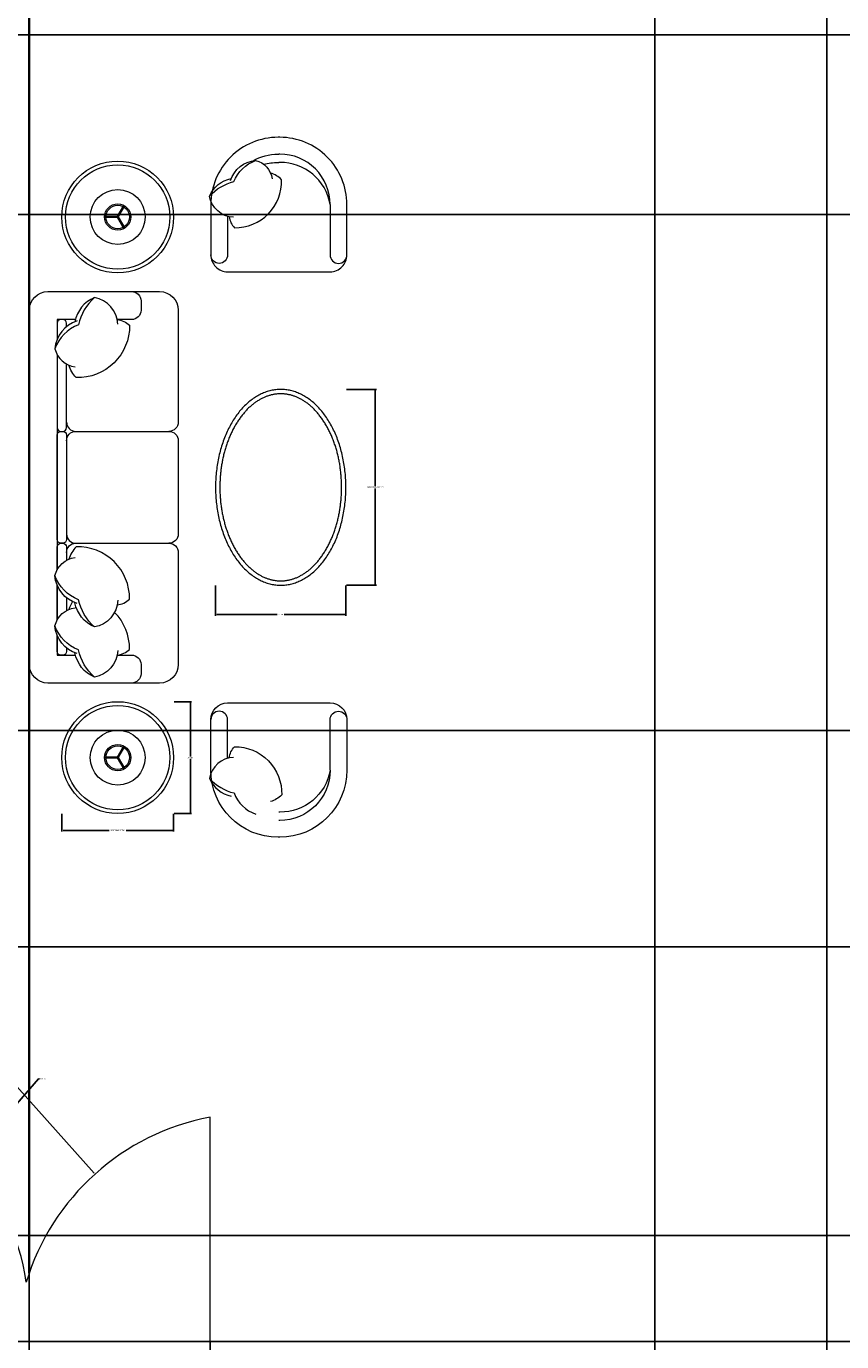
# Model space of a CAD drawing. Units: inches. Extents: x 1861 to 2564, y 1482 to 2317.
# Tile 8 of 11: x 2217 to 2339, y 1853 to 2051. Entities that reach past the tile are written whole.
import ezdxf

# ---------------------------------------------------------------- set-up
doc = ezdxf.new("R2010")
doc.units = ezdxf.units.IN
for name, color, linetype, lineweight in [('A-ANNO-DIMS', 2, 'Continuous', 18), ('A-DOOR', 3, 'Continuous', 18), ('A-FURN', 8, 'Continuous', 13), ('A-WALL', 7, 'Continuous', 35)]:
    doc.layers.add(name, color=color, linetype=linetype, lineweight=lineweight)
doc.styles.get("Standard").update_dxf_attribs({"font": 'arial.ttf'})
doc.dimstyles.get("Standard").update_dxf_attribs({"dimtxt": 0.18, "dimasz": 0.18, "dimexe": 0.18, "dimexo": 0.0625, "dimgap": 0.09, "dimtad": 0, "dimtih": 1, "dimtoh": 1, "dimdec": 4, "dimzin": 0, "dimdsep": 46, "dimtxsty": 'Standard', "dimcen": 0.09, "dimadec": 0, "dimazin": 0, "dimtfac": 1, "dimtdec": 4, "dimtofl": 0, "dimtmove": 0, "dimatfit": 3, "dimfxl": 1, "dimtolj": 1, "dimtzin": 0, "dimarcsym": 0})

# ---------------------------------------------------------------- blocks, each defined once
blk = doc.blocks.new('TABLE-SIDE-ROUND')
at = {"ltscale": 0.03}
for p, q in [((8.34, 8.45), (9.33, 10.16)), ((8.49, 8.36), (9.48, 10.08)), ((8.41, 8.5), (6.44, 8.5)), ((8.41, 8.32), (6.44, 8.32)), ((8.34, 8.36), (9.33, 6.65)), ((8.49, 8.45), (9.48, 6.74))]:
    blk.add_line(p, q, dxfattribs=at)
for radius in [8.41, 4.13, 1.98, 1.77]:
    blk.add_circle((8.41, 8.41), radius, dxfattribs=at)
blk.add_circle((8.41, 8.41), 7.85)
blk = doc.blocks.new('CHAIR-LOUNGE')
at = {"ltscale": 0.03}
blk.add_lwpolyline([(10.44, 0), (18.15, 0, 0.414214), (20.68, 2.53), (20.68, 10.11, 0.414214), (10.57, 20.22), (10.44, 20.22), (10.32, 20.22, 0.414214), (0.21, 10.11), (0.21, 2.53, 0.414214), (2.73, 0), (10.44, 0)], format="xyb", dxfattribs=at)
for points in [[(0, 11.38, -0.14773), (3.69, 13.56, -0.213343), (6.95, 16.74, -0.178662)], [(3.18, 13.73, -0.306663), (6.95, 16.74, -0.30633), (9.42, 13.99, 0.872847)], [(6.55, 16.69, -0.130591), (10.32, 17.69), (10.44, 17.69)], [(8.16, 16.16, -0.072384), (10.32, 16.43), (10.44, 16.43)], [(18.15, 10.11, 0.414214), (10.57, 17.69), (10.44, 17.69)], [(18.15, 10.11, 0.372719), (10.57, 16.43), (10.44, 16.43)], [(3.62, 8.2, -0.356772), (0, 11.38, -0.249542), (3.28, 14.01, 9.61688)], [(2.98, 8.28, 0.165541), (3.77, 6.61, 0.425989), (10.86, 13.85, 0.121523), (9.18, 14.84, -7.115464)], [(18.15, 10.11), (18.15, 2.53, 0.414214), (19.42, 1.26), (19.42, 1.26, 0.414214), (20.68, 2.53)], [(2.73, 8.34), (2.73, 2.53, -0.414214), (1.47, 1.26), (1.47, 1.26, -0.414214), (0.21, 2.53)]]:
    blk.add_lwpolyline(points, format="xyb")
blk = doc.blocks.new('TABLE-COFFEE-OVAL')
at = {"ltscale": 0.03}
blk.add_polyline3d([(9.81, 29.44, 0), (9.63, 29.44, 0), (9.44, 29.43, 0), (9.26, 29.41, 0), (9.07, 29.4, 0), (8.89, 29.37, 0), (8.7, 29.34, 0), (8.52, 29.31, 0), (8.33, 29.27, 0), (8.15, 29.23, 0), (7.97, 29.18, 0), (7.79, 29.12, 0), (7.6, 29.06, 0), (7.42, 28.99, 0), (7.24, 28.92, 0), (7.07, 28.85, 0), (6.89, 28.77, 0), (6.71, 28.68, 0), (6.54, 28.59, 0), (6.36, 28.5, 0), (6.19, 28.4, 0), (6.02, 28.29, 0), (5.85, 28.18, 0), (5.68, 28.07, 0), (5.51, 27.95, 0), (5.34, 27.82, 0), (5.18, 27.69, 0), (5.02, 27.56, 0), (4.85, 27.42, 0), (4.69, 27.28, 0), (4.54, 27.13, 0), (4.38, 26.98, 0), (4.23, 26.82, 0), (4.08, 26.66, 0), (3.93, 26.49, 0), (3.78, 26.33, 0), (3.63, 26.15, 0), (3.49, 25.97, 0), (3.35, 25.79, 0), (3.21, 25.61, 0), (3.08, 25.42, 0), (2.94, 25.23, 0), (2.81, 25.03, 0), (2.68, 24.83, 0), (2.56, 24.62, 0), (2.43, 24.42, 0), (2.31, 24.2, 0), (2.19, 23.99, 0), (2.08, 23.77, 0), (1.96, 23.55, 0), (1.85, 23.33, 0), (1.75, 23.1, 0), (1.64, 22.87, 0), (1.54, 22.63, 0), (1.44, 22.4, 0), (1.35, 22.16, 0), (1.26, 21.92, 0), (1.17, 21.67, 0), (1.08, 21.43, 0), (1, 21.18, 0), (0.92, 20.93, 0), (0.84, 20.67, 0), (0.77, 20.42, 0), (0.7, 20.16, 0), (0.63, 19.9, 0), (0.57, 19.64, 0), (0.51, 19.37, 0), (0.45, 19.11, 0), (0.39, 18.84, 0), (0.34, 18.57, 0), (0.3, 18.31, 0), (0.25, 18.03, 0), (0.21, 17.76, 0), (0.18, 17.49, 0), (0.14, 17.22, 0), (0.11, 16.94, 0), (0.09, 16.66, 0), (0.07, 16.39, 0), (0.05, 16.11, 0), (0.03, 15.83, 0), (0.02, 15.56, 0), (0.01, 15.28, 0), (0, 15, 0), (0, 14.72, 0), (0, 14.44, 0), (0.01, 14.16, 0), (0.02, 13.89, 0), (0.03, 13.61, 0), (0.05, 13.33, 0), (0.07, 13.05, 0), (0.09, 12.78, 0), (0.11, 12.5, 0), (0.14, 12.23, 0), (0.18, 11.95, 0), (0.21, 11.68, 0), (0.25, 11.41, 0), (0.3, 11.14, 0), (0.34, 10.87, 0), (0.39, 10.6, 0), (0.45, 10.33, 0), (0.51, 10.07, 0), (0.57, 9.8, 0), (0.63, 9.54, 0), (0.7, 9.28, 0), (0.77, 9.02, 0), (0.84, 8.77, 0), (0.92, 8.52, 0), (1, 8.26, 0), (1.08, 8.01, 0), (1.17, 7.77, 0), (1.26, 7.52, 0), (1.35, 7.28, 0), (1.44, 7.04, 0), (1.54, 6.81, 0), (1.64, 6.57, 0), (1.75, 6.34, 0), (1.85, 6.12, 0), (1.96, 5.89, 0), (2.08, 5.67, 0), (2.19, 5.45, 0), (2.31, 5.24, 0), (2.43, 5.03, 0), (2.56, 4.82, 0), (2.68, 4.61, 0), (2.81, 4.41, 0), (2.94, 4.22, 0), (3.08, 4.02, 0), (3.21, 3.83, 0), (3.35, 3.65, 0), (3.49, 3.47, 0), (3.63, 3.29, 0), (3.78, 3.12, 0), (3.93, 2.95, 0), (4.08, 2.78, 0), (4.23, 2.62, 0), (4.38, 2.46, 0), (4.54, 2.31, 0), (4.69, 2.17, 0), (4.85, 2.02, 0), (5.02, 1.88, 0), (5.18, 1.75, 0), (5.34, 1.62, 0), (5.51, 1.5, 0), (5.68, 1.38, 0), (5.85, 1.26, 0), (6.02, 1.15, 0), (6.19, 1.05, 0), (6.36, 0.94, 0), (6.54, 0.85, 0), (6.71, 0.76, 0), (6.89, 0.67, 0), (7.07, 0.59, 0), (7.24, 0.52, 0), (7.42, 0.45, 0), (7.6, 0.38, 0), (7.79, 0.32, 0), (7.97, 0.27, 0), (8.15, 0.22, 0), (8.33, 0.17, 0), (8.52, 0.13, 0), (8.7, 0.1, 0), (8.89, 0.07, 0), (9.07, 0.05, 0), (9.26, 0.03, 0), (9.44, 0.01, 0), (9.63, 0.01, 0), (9.81, 0, 0), (10, 0.01, 0), (10.18, 0.01, 0), (10.37, 0.03, 0), (10.56, 0.05, 0), (10.74, 0.07, 0), (10.93, 0.1, 0), (11.11, 0.13, 0), (11.29, 0.17, 0), (11.48, 0.22, 0), (11.66, 0.27, 0), (11.84, 0.32, 0), (12.02, 0.38, 0), (12.2, 0.45, 0), (12.38, 0.52, 0), (12.56, 0.59, 0), (12.74, 0.67, 0), (12.92, 0.76, 0), (13.09, 0.85, 0), (13.27, 0.94, 0), (13.44, 1.05, 0), (13.61, 1.15, 0), (13.78, 1.26, 0), (13.95, 1.38, 0), (14.12, 1.5, 0), (14.28, 1.62, 0), (14.45, 1.75, 0), (14.61, 1.88, 0), (14.77, 2.02, 0), (14.93, 2.17, 0), (15.09, 2.31, 0), (15.25, 2.46, 0), (15.4, 2.62, 0), (15.55, 2.78, 0), (15.7, 2.95, 0), (15.85, 3.12, 0), (15.99, 3.29, 0), (16.14, 3.47, 0), (16.28, 3.65, 0), (16.42, 3.83, 0), (16.55, 4.02, 0), (16.69, 4.22, 0), (16.82, 4.41, 0), (16.95, 4.61, 0), (17.07, 4.82, 0), (17.2, 5.03, 0), (17.32, 5.24, 0), (17.43, 5.45, 0), (17.55, 5.67, 0), (17.66, 5.89, 0), (17.77, 6.12, 0), (17.88, 6.34, 0), (17.98, 6.57, 0), (18.09, 6.81, 0), (18.18, 7.04, 0), (18.28, 7.28, 0), (18.37, 7.52, 0), (18.46, 7.77, 0), (18.55, 8.01, 0), (18.63, 8.26, 0), (18.71, 8.52, 0), (18.79, 8.77, 0), (18.86, 9.02, 0), (18.93, 9.28, 0), (19, 9.54, 0), (19.06, 9.8, 0), (19.12, 10.07, 0), (19.18, 10.33, 0), (19.23, 10.6, 0), (19.28, 10.87, 0), (19.33, 11.14, 0), (19.37, 11.41, 0), (19.41, 11.68, 0), (19.45, 11.95, 0), (19.48, 12.23, 0), (19.51, 12.5, 0), (19.54, 12.78, 0), (19.56, 13.05, 0), (19.58, 13.33, 0), (19.6, 13.61, 0), (19.61, 13.89, 0), (19.62, 14.16, 0), (19.62, 14.44, 0), (19.63, 14.72, 0), (19.62, 15, 0), (19.62, 15.28, 0), (19.61, 15.56, 0), (19.6, 15.83, 0), (19.58, 16.11, 0), (19.56, 16.39, 0), (19.54, 16.66, 0), (19.51, 16.94, 0), (19.48, 17.22, 0), (19.45, 17.49, 0), (19.41, 17.76, 0), (19.37, 18.03, 0), (19.33, 18.31, 0), (19.28, 18.57, 0), (19.23, 18.84, 0), (19.18, 19.11, 0), (19.12, 19.37, 0), (19.06, 19.64, 0), (19, 19.9, 0), (18.93, 20.16, 0), (18.86, 20.42, 0), (18.79, 20.67, 0), (18.71, 20.93, 0), (18.63, 21.18, 0), (18.55, 21.43, 0), (18.46, 21.67, 0), (18.37, 21.92, 0), (18.28, 22.16, 0), (18.18, 22.4, 0), (18.09, 22.63, 0), (17.98, 22.87, 0), (17.88, 23.1, 0), (17.77, 23.33, 0), (17.66, 23.55, 0), (17.55, 23.77, 0), (17.43, 23.99, 0), (17.32, 24.2, 0), (17.2, 24.42, 0), (17.07, 24.62, 0), (16.95, 24.83, 0), (16.82, 25.03, 0), (16.69, 25.23, 0), (16.55, 25.42, 0), (16.42, 25.61, 0), (16.28, 25.79, 0), (16.14, 25.97, 0), (15.99, 26.15, 0), (15.85, 26.33, 0), (15.7, 26.49, 0), (15.55, 26.66, 0), (15.4, 26.82, 0), (15.25, 26.98, 0), (15.09, 27.13, 0), (14.93, 27.28, 0), (14.77, 27.42, 0), (14.61, 27.56, 0), (14.45, 27.69, 0), (14.28, 27.82, 0), (14.12, 27.95, 0), (13.95, 28.07, 0), (13.78, 28.18, 0), (13.61, 28.29, 0), (13.44, 28.4, 0), (13.27, 28.5, 0), (13.09, 28.59, 0), (12.92, 28.68, 0), (12.74, 28.77, 0), (12.56, 28.85, 0), (12.38, 28.92, 0), (12.2, 28.99, 0), (12.02, 29.06, 0), (11.84, 29.12, 0), (11.66, 29.18, 0), (11.48, 29.23, 0), (11.29, 29.27, 0), (11.11, 29.31, 0), (10.93, 29.34, 0), (10.74, 29.37, 0), (10.56, 29.4, 0), (10.37, 29.41, 0), (10.18, 29.43, 0), (10, 29.44, 0), (9.81, 29.44, 0)], dxfattribs=at)
blk.add_polyline3d([(9.81, 28.78, 0), (9.71, 28.78, 0), (9.61, 28.78, 0), (9.51, 28.78, 0), (9.41, 28.77, 0), (9.31, 28.76, 0), (9.2, 28.75, 0), (9.1, 28.74, 0), (9, 28.73, 0), (8.89, 28.71, 0), (8.79, 28.69, 0), (8.69, 28.68, 0), (8.58, 28.65, 0), (8.48, 28.63, 0), (8.37, 28.61, 0), (8.27, 28.58, 0), (8.16, 28.55, 0), (8.05, 28.52, 0), (7.95, 28.49, 0), (7.84, 28.45, 0), (7.73, 28.41, 0), (7.63, 28.37, 0), (7.52, 28.33, 0), (7.41, 28.29, 0), (7.31, 28.24, 0), (7.2, 28.19, 0), (7.09, 28.14, 0), (6.98, 28.09, 0), (6.88, 28.03, 0), (6.77, 27.97, 0), (6.66, 27.91, 0), (6.55, 27.85, 0), (6.45, 27.79, 0), (6.34, 27.72, 0), (6.23, 27.65, 0), (6.13, 27.58, 0), (6.02, 27.51, 0), (5.92, 27.43, 0), (5.81, 27.36, 0), (5.71, 27.28, 0), (5.6, 27.19, 0), (5.5, 27.11, 0), (5.39, 27.02, 0), (5.29, 26.93, 0), (5.19, 26.84, 0), (5.09, 26.75, 0), (4.98, 26.65, 0), (4.88, 26.55, 0), (4.78, 26.45, 0), (4.68, 26.34, 0), (4.58, 26.24, 0), (4.49, 26.13, 0), (4.39, 26.02, 0), (4.29, 25.91, 0), (4.2, 25.79, 0), (4.1, 25.68, 0), (4.01, 25.56, 0), (3.91, 25.44, 0), (3.82, 25.32, 0), (3.73, 25.19, 0), (3.64, 25.07, 0), (3.55, 24.94, 0), (3.46, 24.81, 0), (3.37, 24.68, 0), (3.29, 24.54, 0), (3.2, 24.41, 0), (3.12, 24.27, 0), (3.03, 24.13, 0), (2.95, 23.99, 0), (2.87, 23.85, 0), (2.79, 23.71, 0), (2.71, 23.56, 0), (2.63, 23.41, 0), (2.56, 23.27, 0), (2.48, 23.12, 0), (2.41, 22.97, 0), (2.34, 22.81, 0), (2.27, 22.66, 0), (2.2, 22.51, 0), (2.13, 22.35, 0), (2.07, 22.19, 0), (2, 22.04, 0), (1.94, 21.88, 0), (1.88, 21.72, 0), (1.82, 21.55, 0), (1.76, 21.39, 0), (1.7, 21.23, 0), (1.65, 21.07, 0), (1.6, 20.9, 0), (1.54, 20.74, 0), (1.49, 20.58, 0), (1.44, 20.41, 0), (1.4, 20.25, 0), (1.35, 20.08, 0), (1.31, 19.92, 0), (1.26, 19.75, 0), (1.22, 19.59, 0), (1.18, 19.42, 0), (1.15, 19.25, 0), (1.11, 19.09, 0), (1.07, 18.92, 0), (1.04, 18.75, 0), (1.01, 18.58, 0), (0.98, 18.42, 0), (0.95, 18.25, 0), (0.92, 18.08, 0), (0.89, 17.91, 0), (0.87, 17.74, 0), (0.84, 17.57, 0), (0.82, 17.4, 0), (0.8, 17.23, 0), (0.78, 17.06, 0), (0.76, 16.89, 0), (0.75, 16.72, 0), (0.73, 16.55, 0), (0.72, 16.38, 0), (0.71, 16.21, 0), (0.7, 16.04, 0), (0.69, 15.87, 0), (0.68, 15.7, 0), (0.67, 15.53, 0), (0.67, 15.36, 0), (0.66, 15.19, 0), (0.66, 15.02, 0), (0.66, 14.85, 0), (0.66, 14.68, 0), (0.66, 14.51, 0), (0.66, 14.34, 0), (0.66, 14.17, 0), (0.67, 14, 0), (0.67, 13.82, 0), (0.68, 13.65, 0), (0.69, 13.48, 0), (0.7, 13.31, 0), (0.71, 13.14, 0), (0.73, 12.97, 0), (0.74, 12.8, 0), (0.76, 12.63, 0), (0.77, 12.46, 0), (0.79, 12.29, 0), (0.81, 12.12, 0), (0.83, 11.95, 0), (0.86, 11.78, 0), (0.88, 11.62, 0), (0.91, 11.45, 0), (0.93, 11.28, 0), (0.96, 11.11, 0), (0.99, 10.94, 0), (1.02, 10.77, 0), (1.06, 10.61, 0), (1.09, 10.44, 0), (1.13, 10.27, 0), (1.16, 10.1, 0), (1.2, 9.94, 0), (1.24, 9.77, 0), (1.29, 9.61, 0), (1.33, 9.44, 0), (1.37, 9.28, 0), (1.42, 9.11, 0), (1.47, 8.95, 0), (1.52, 8.78, 0), (1.57, 8.62, 0), (1.62, 8.46, 0), (1.68, 8.29, 0), (1.73, 8.13, 0), (1.79, 7.97, 0), (1.85, 7.81, 0), (1.91, 7.65, 0), (1.97, 7.49, 0), (2.03, 7.33, 0), (2.1, 7.17, 0), (2.17, 7.01, 0), (2.23, 6.86, 0), (2.3, 6.7, 0), (2.37, 6.55, 0), (2.45, 6.4, 0), (2.52, 6.25, 0), (2.6, 6.1, 0), (2.67, 5.95, 0), (2.75, 5.81, 0), (2.83, 5.66, 0), (2.91, 5.52, 0), (2.99, 5.38, 0), (3.07, 5.24, 0), (3.16, 5.1, 0), (3.24, 4.97, 0), (3.33, 4.83, 0), (3.42, 4.7, 0), (3.5, 4.57, 0), (3.59, 4.44, 0), (3.68, 4.31, 0), (3.77, 4.19, 0), (3.87, 4.06, 0), (3.96, 3.94, 0), (4.05, 3.82, 0), (4.15, 3.71, 0), (4.24, 3.59, 0), (4.34, 3.48, 0), (4.44, 3.37, 0), (4.53, 3.26, 0), (4.63, 3.15, 0), (4.73, 3.04, 0), (4.83, 2.94, 0), (4.93, 2.84, 0), (5.03, 2.74, 0), (5.14, 2.65, 0), (5.24, 2.56, 0), (5.34, 2.47, 0), (5.44, 2.38, 0), (5.55, 2.29, 0), (5.65, 2.21, 0), (5.76, 2.13, 0), (5.86, 2.05, 0), (5.97, 1.97, 0), (6.07, 1.9, 0), (6.18, 1.82, 0), (6.29, 1.75, 0), (6.39, 1.69, 0), (6.5, 1.62, 0), (6.61, 1.56, 0), (6.72, 1.5, 0), (6.82, 1.44, 0), (6.93, 1.38, 0), (7.04, 1.33, 0), (7.14, 1.28, 0), (7.25, 1.23, 0), (7.36, 1.18, 0), (7.47, 1.13, 0), (7.57, 1.09, 0), (7.68, 1.05, 0), (7.79, 1.01, 0), (7.89, 0.97, 0), (8, 0.94, 0), (8.11, 0.91, 0), (8.21, 0.88, 0), (8.32, 0.85, 0), (8.42, 0.82, 0), (8.53, 0.8, 0), (8.63, 0.78, 0), (8.74, 0.76, 0), (8.84, 0.74, 0), (8.95, 0.72, 0), (9.05, 0.71, 0), (9.15, 0.69, 0), (9.26, 0.68, 0), (9.36, 0.68, 0), (9.46, 0.67, 0), (9.56, 0.66, 0), (9.66, 0.66, 0), (9.76, 0.66, 0), (9.86, 0.66, 0), (9.96, 0.66, 0), (10.07, 0.66, 0), (10.17, 0.67, 0), (10.27, 0.68, 0), (10.37, 0.68, 0), (10.47, 0.69, 0), (10.58, 0.71, 0), (10.68, 0.72, 0), (10.78, 0.74, 0), (10.89, 0.76, 0), (10.99, 0.78, 0), (11.1, 0.8, 0), (11.2, 0.82, 0), (11.31, 0.85, 0), (11.41, 0.88, 0), (11.52, 0.91, 0), (11.63, 0.94, 0), (11.73, 0.97, 0), (11.84, 1.01, 0), (11.95, 1.05, 0), (12.05, 1.09, 0), (12.16, 1.13, 0), (12.27, 1.18, 0), (12.37, 1.23, 0), (12.48, 1.28, 0), (12.59, 1.33, 0), (12.7, 1.38, 0), (12.8, 1.44, 0), (12.91, 1.5, 0), (13.02, 1.56, 0), (13.13, 1.62, 0), (13.23, 1.69, 0), (13.34, 1.75, 0), (13.45, 1.82, 0), (13.55, 1.9, 0), (13.66, 1.97, 0), (13.76, 2.05, 0), (13.87, 2.13, 0), (13.97, 2.21, 0), (14.08, 2.29, 0), (14.18, 2.38, 0), (14.29, 2.47, 0), (14.39, 2.56, 0), (14.49, 2.65, 0), (14.59, 2.74, 0), (14.69, 2.84, 0), (14.79, 2.94, 0), (14.89, 3.04, 0), (14.99, 3.15, 0), (15.09, 3.26, 0), (15.19, 3.37, 0), (15.29, 3.48, 0), (15.38, 3.59, 0), (15.48, 3.71, 0), (15.57, 3.82, 0), (15.67, 3.94, 0), (15.76, 4.06, 0), (15.85, 4.19, 0), (15.94, 4.31, 0), (16.03, 4.44, 0), (16.12, 4.57, 0), (16.21, 4.7, 0), (16.3, 4.83, 0), (16.38, 4.97, 0), (16.47, 5.1, 0), (16.55, 5.24, 0), (16.64, 5.38, 0), (16.72, 5.52, 0), (16.8, 5.66, 0), (16.88, 5.81, 0), (16.95, 5.95, 0), (17.03, 6.1, 0), (17.11, 6.25, 0), (17.18, 6.4, 0), (17.25, 6.55, 0), (17.32, 6.7, 0), (17.39, 6.86, 0), (17.46, 7.01, 0), (17.53, 7.17, 0), (17.59, 7.33, 0), (17.66, 7.49, 0), (17.72, 7.65, 0), (17.78, 7.81, 0), (17.84, 7.97, 0), (17.9, 8.13, 0), (17.95, 8.29, 0), (18.01, 8.46, 0), (18.06, 8.62, 0), (18.11, 8.78, 0), (18.16, 8.95, 0), (18.21, 9.11, 0), (18.25, 9.28, 0), (18.3, 9.44, 0), (18.34, 9.61, 0), (18.38, 9.77, 0), (18.42, 9.94, 0), (18.46, 10.1, 0), (18.5, 10.27, 0), (18.54, 10.44, 0), (18.57, 10.61, 0), (18.6, 10.77, 0), (18.63, 10.94, 0), (18.66, 11.11, 0), (18.69, 11.28, 0), (18.72, 11.45, 0), (18.75, 11.62, 0), (18.77, 11.78, 0), (18.79, 11.95, 0), (18.81, 12.12, 0), (18.83, 12.29, 0), (18.85, 12.46, 0), (18.87, 12.63, 0), (18.89, 12.8, 0), (18.9, 12.97, 0), (18.91, 13.14, 0), (18.93, 13.31, 0), (18.94, 13.48, 0), (18.95, 13.65, 0), (18.95, 13.82, 0), (18.96, 14, 0), (18.96, 14.17, 0), (18.97, 14.34, 0), (18.97, 14.51, 0), (18.97, 14.68, 0), (18.97, 14.85, 0), (18.97, 15.02, 0), (18.97, 15.19, 0), (18.96, 15.36, 0), (18.96, 15.53, 0), (18.95, 15.7, 0), (18.94, 15.87, 0), (18.93, 16.04, 0), (18.92, 16.21, 0), (18.91, 16.38, 0), (18.89, 16.55, 0), (18.88, 16.72, 0), (18.86, 16.89, 0), (18.84, 17.06, 0), (18.83, 17.23, 0), (18.8, 17.4, 0), (18.78, 17.57, 0), (18.76, 17.74, 0), (18.73, 17.91, 0), (18.71, 18.08, 0), (18.68, 18.25, 0), (18.65, 18.42, 0), (18.62, 18.58, 0), (18.59, 18.75, 0), (18.55, 18.92, 0), (18.52, 19.09, 0), (18.48, 19.25, 0), (18.44, 19.42, 0), (18.4, 19.59, 0), (18.36, 19.75, 0), (18.32, 19.92, 0), (18.28, 20.08, 0), (18.23, 20.25, 0), (18.18, 20.41, 0), (18.13, 20.58, 0), (18.08, 20.74, 0), (18.03, 20.9, 0), (17.98, 21.07, 0), (17.92, 21.23, 0), (17.87, 21.39, 0), (17.81, 21.55, 0), (17.75, 21.72, 0), (17.69, 21.88, 0), (17.62, 22.04, 0), (17.56, 22.19, 0), (17.49, 22.35, 0), (17.43, 22.51, 0), (17.36, 22.66, 0), (17.29, 22.81, 0), (17.22, 22.97, 0), (17.14, 23.12, 0), (17.07, 23.27, 0), (16.99, 23.41, 0), (16.92, 23.56, 0), (16.84, 23.71, 0), (16.76, 23.85, 0), (16.68, 23.99, 0), (16.59, 24.13, 0), (16.51, 24.27, 0), (16.43, 24.41, 0), (16.34, 24.54, 0), (16.26, 24.68, 0), (16.17, 24.81, 0), (16.08, 24.94, 0), (15.99, 25.07, 0), (15.9, 25.19, 0), (15.81, 25.32, 0), (15.71, 25.44, 0), (15.62, 25.56, 0), (15.53, 25.68, 0), (15.43, 25.79, 0), (15.34, 25.91, 0), (15.24, 26.02, 0), (15.14, 26.13, 0), (15.04, 26.24, 0), (14.94, 26.34, 0), (14.84, 26.45, 0), (14.74, 26.55, 0), (14.64, 26.65, 0), (14.54, 26.75, 0), (14.44, 26.84, 0), (14.34, 26.93, 0), (14.23, 27.02, 0), (14.13, 27.11, 0), (14.03, 27.19, 0), (13.92, 27.28, 0), (13.82, 27.36, 0), (13.71, 27.43, 0), (13.61, 27.51, 0), (13.5, 27.58, 0), (13.39, 27.65, 0), (13.29, 27.72, 0), (13.18, 27.79, 0), (13.07, 27.85, 0), (12.97, 27.91, 0), (12.86, 27.97, 0), (12.75, 28.03, 0), (12.64, 28.09, 0), (12.54, 28.14, 0), (12.43, 28.19, 0), (12.32, 28.24, 0), (12.21, 28.29, 0), (12.11, 28.33, 0), (12, 28.37, 0), (11.89, 28.41, 0), (11.79, 28.45, 0), (11.68, 28.49, 0), (11.57, 28.52, 0), (11.47, 28.55, 0), (11.36, 28.58, 0), (11.26, 28.61, 0), (11.15, 28.63, 0), (11.05, 28.65, 0), (10.94, 28.68, 0), (10.84, 28.69, 0), (10.73, 28.71, 0), (10.63, 28.73, 0), (10.53, 28.74, 0), (10.42, 28.75, 0), (10.32, 28.76, 0), (10.22, 28.77, 0), (10.12, 28.78, 0), (10.01, 28.78, 0), (9.91, 28.78, 0), (9.81, 28.78, 0)])
blk = doc.blocks.new('*D28')
at = {"layer": 'A-ANNO-DIMS', "color": 0, "lineweight": -2, "transparency": 16777216}
for p, q in [((2222.15, 1932.74), (2222.15, 1930.1)), ((2238.96, 1932.74), (2238.96, 1930.1)), ((2222.33, 1930.28), (2229.27, 1930.28)), ((2238.78, 1930.28), (2231.84, 1930.28))]:
    blk.add_line(p, q, dxfattribs=at)
at = {"layer": 'A-ANNO-DIMS', "color": 0, "transparency": 16777216}
for points in [[(2222.33, 1930.31), (2222.33, 1930.25), (2222.15, 1930.28)], [(2238.78, 1930.31), (2238.78, 1930.25), (2238.96, 1930.28)]]:
    blk.add_solid(points, dxfattribs=at)
at = {"layer": 'Defpoints', "color": 0, "transparency": 16777216}
for p in [(2222.15, 1932.8), (2238.96, 1932.8), (2238.96, 1930.28)]:
    blk.add_point(p, dxfattribs=at)
at = {"layer": 'A-ANNO-DIMS', "color": 0, "transparency": 16777216, "insert": (2230.55, 1930.28), "char_height": 0.18, "attachment_point": 5}
blk.add_mtext('\\A1;SIDE TABLE 17 TYP.', dxfattribs=at)
blk = doc.blocks.new('*D29')
at = {"layer": 'A-ANNO-DIMS', "color": 0, "lineweight": -2, "transparency": 16777216}
for p, q in [((2239.03, 1949.62), (2241.67, 1949.62)), ((2241.49, 1949.44), (2241.49, 1941.39)), ((2241.49, 1932.98), (2241.49, 1941.03)), ((2239.03, 1932.8), (2241.67, 1932.8))]:
    blk.add_line(p, q, dxfattribs=at)
at = {"layer": 'A-ANNO-DIMS', "color": 0, "transparency": 16777216}
for points in [[(2241.46, 1949.44), (2241.52, 1949.44), (2241.49, 1949.62)], [(2241.46, 1932.98), (2241.52, 1932.98), (2241.49, 1932.8)]]:
    blk.add_solid(points, dxfattribs=at)
at = {"layer": 'Defpoints', "color": 0, "transparency": 16777216}
for p in [(2238.96, 1949.62), (2241.49, 1949.62), (2238.96, 1932.8)]:
    blk.add_point(p, dxfattribs=at)
at = {"layer": 'A-ANNO-DIMS', "color": 0, "transparency": 16777216, "insert": (2241.49, 1941.21), "char_height": 0.18, "attachment_point": 5}
blk.add_mtext('\\A1;17 TYP.', dxfattribs=at)
blk = doc.blocks.new('*D30')
at = {"layer": 'A-ANNO-DIMS', "color": 0, "lineweight": -2, "transparency": 16777216}
for p, q in [((2264.96, 1996.58), (2269.49, 1996.58)), ((2269.31, 1996.4), (2269.31, 1982.04)), ((2269.31, 1967.32), (2269.31, 1981.68)), ((2264.96, 1967.14), (2269.49, 1967.14))]:
    blk.add_line(p, q, dxfattribs=at)
at = {"layer": 'A-ANNO-DIMS', "color": 0, "transparency": 16777216}
for points in [[(2269.28, 1996.4), (2269.34, 1996.4), (2269.31, 1996.58)], [(2269.28, 1967.32), (2269.34, 1967.32), (2269.31, 1967.14)]]:
    blk.add_solid(points, dxfattribs=at)
at = {"layer": 'Defpoints', "color": 0, "transparency": 16777216}
for p in [(2264.9, 1996.58), (2269.31, 1996.58), (2264.9, 1967.14)]:
    blk.add_point(p, dxfattribs=at)
at = {"layer": 'A-ANNO-DIMS', "color": 0, "transparency": 16777216, "insert": (2269.31, 1981.86), "char_height": 0.18, "attachment_point": 5}
blk.add_mtext('\\A1;COFFEE TABLE 29 TYP.', dxfattribs=at)
blk = doc.blocks.new('*D31')
at = {"layer": 'A-ANNO-DIMS', "color": 0, "lineweight": -2, "transparency": 16777216}
for p, q in [((2245.27, 1967.08), (2245.27, 1962.55)), ((2264.9, 1967.08), (2264.9, 1962.55)), ((2245.45, 1962.73), (2254.55, 1962.73)), ((2264.72, 1962.73), (2255.61, 1962.73))]:
    blk.add_line(p, q, dxfattribs=at)
at = {"layer": 'A-ANNO-DIMS', "color": 0, "transparency": 16777216}
for points in [[(2245.45, 1962.76), (2245.45, 1962.7), (2245.27, 1962.73)], [(2264.72, 1962.76), (2264.72, 1962.7), (2264.9, 1962.73)]]:
    blk.add_solid(points, dxfattribs=at)
at = {"layer": 'Defpoints', "color": 0, "transparency": 16777216}
for p in [(2245.27, 1967.14), (2264.9, 1967.14), (2264.9, 1962.73)]:
    blk.add_point(p, dxfattribs=at)
at = {"layer": 'A-ANNO-DIMS', "color": 0, "transparency": 16777216, "insert": (2255.08, 1962.73), "char_height": 0.18, "attachment_point": 5}
blk.add_mtext('\\A1;20 TYP.', dxfattribs=at)
blk = doc.blocks.new('*D37')
at = {"layer": 'A-ANNO-DIMS', "color": 0, "lineweight": -2, "transparency": 16777216}
for p, q in [((2311.38, 2250.82), (2311.38, 1545.6)), ((2337.24, 2250.82), (2337.24, 1545.6)), ((2311.56, 1545.78), (2323.91, 1545.78)), ((2337.06, 1545.78), (2324.7, 1545.78))]:
    blk.add_line(p, q, dxfattribs=at)
at = {"layer": 'A-ANNO-DIMS', "color": 0, "transparency": 16777216}
for points in [[(2311.56, 1545.81), (2311.56, 1545.75), (2311.38, 1545.78)], [(2337.06, 1545.81), (2337.06, 1545.75), (2337.24, 1545.78)]]:
    blk.add_solid(points, dxfattribs=at)
at = {"layer": 'Defpoints', "color": 0, "transparency": 16777216}
for p in [(2311.38, 2250.89), (2337.24, 2250.89), (2337.24, 1545.78)]:
    blk.add_point(p, dxfattribs=at)
at = {"layer": 'A-ANNO-DIMS', "color": 0, "transparency": 16777216, "insert": (2324.31, 1545.78), "char_height": 0.18, "attachment_point": 5}
blk.add_mtext('\\A1;25.86', dxfattribs=at)
blk = doc.blocks.new('*D53')
at = {"layer": 'A-ANNO-DIMS', "color": 0, "lineweight": -2, "transparency": 16777216}
for p, q in [((2076.3, 1945.29), (2537.22, 1945.29)), ((2537.04, 1945.11), (2537.04, 1929.2)), ((2537.04, 1912.93), (2537.04, 1928.84)), ((2076.3, 1912.75), (2537.22, 1912.75))]:
    blk.add_line(p, q, dxfattribs=at)
at = {"layer": 'A-ANNO-DIMS', "color": 0, "transparency": 16777216}
for points in [[(2537.01, 1945.11), (2537.07, 1945.11), (2537.04, 1945.29)], [(2537.01, 1912.93), (2537.07, 1912.93), (2537.04, 1912.75)]]:
    blk.add_solid(points, dxfattribs=at)
at = {"layer": 'Defpoints', "color": 0, "transparency": 16777216}
for p in [(2076.24, 1945.29), (2537.04, 1945.29), (2076.24, 1912.75)]:
    blk.add_point(p, dxfattribs=at)
at = {"layer": 'A-ANNO-DIMS', "color": 0, "transparency": 16777216, "insert": (2537.04, 1929.02), "char_height": 0.18, "attachment_point": 5}
blk.add_mtext('\\A1;32.544', dxfattribs=at)
blk = doc.blocks.new('*D56')
at = {"layer": 'A-ANNO-DIMS', "color": 0, "lineweight": -2, "transparency": 16777216}
for p, q in [((2186.51, 1853.32), (2186.51, 1545.6)), ((2244.44, 1853.32), (2244.44, 1545.6)), ((2186.69, 1545.78), (2215.08, 1545.78)), ((2244.26, 1545.78), (2215.87, 1545.78))]:
    blk.add_line(p, q, dxfattribs=at)
at = {"layer": 'A-ANNO-DIMS', "color": 0, "transparency": 16777216}
for points in [[(2186.69, 1545.81), (2186.69, 1545.75), (2186.51, 1545.78)], [(2244.26, 1545.81), (2244.26, 1545.75), (2244.44, 1545.78)]]:
    blk.add_solid(points, dxfattribs=at)
at = {"layer": 'Defpoints', "color": 0, "transparency": 16777216}
for p in [(2186.51, 1853.39), (2244.44, 1853.39), (2244.44, 1545.78)]:
    blk.add_point(p, dxfattribs=at)
at = {"layer": 'A-ANNO-DIMS', "color": 0, "transparency": 16777216, "insert": (2215.48, 1545.78), "char_height": 0.18, "attachment_point": 5}
blk.add_mtext('\\A1;57.93', dxfattribs=at)
blk = doc.blocks.new('*D65')
at = {"layer": 'A-ANNO-DIMS', "color": 0, "lineweight": -2, "transparency": 16777216}
for p, q in [((2497.68, 2049.89), (1892.76, 2049.89)), ((1892.94, 2049.71), (1892.94, 2036.58)), ((1892.94, 2023.09), (1892.94, 2036.22)), ((2497.68, 2022.91), (1892.76, 2022.91))]:
    blk.add_line(p, q, dxfattribs=at)
at = {"layer": 'A-ANNO-DIMS', "color": 0, "transparency": 16777216}
for points in [[(1892.91, 2049.71), (1892.97, 2049.71), (1892.94, 2049.89)], [(1892.91, 2023.09), (1892.97, 2023.09), (1892.94, 2022.91)]]:
    blk.add_solid(points, dxfattribs=at)
at = {"layer": 'Defpoints', "color": 0, "transparency": 16777216}
for p in [(2497.74, 2049.89), (1892.94, 2022.91), (2497.74, 2022.91)]:
    blk.add_point(p, dxfattribs=at)
at = {"layer": 'A-ANNO-DIMS', "color": 0, "transparency": 16777216, "insert": (1892.94, 2036.4), "char_height": 0.18, "attachment_point": 5}
blk.add_mtext('\\A1;26.973', dxfattribs=at)
blk = doc.blocks.new('*D66')
at = {"layer": 'A-ANNO-DIMS', "color": 0, "lineweight": -2, "transparency": 16777216}
for p, q in [((2497.68, 1869.33), (1892.76, 1869.33)), ((1892.94, 1869.15), (1892.94, 1861.54)), ((1892.94, 1853.57), (1892.94, 1861.17)), ((2497.68, 1853.39), (1892.76, 1853.39))]:
    blk.add_line(p, q, dxfattribs=at)
at = {"layer": 'A-ANNO-DIMS', "color": 0, "transparency": 16777216}
for points in [[(1892.91, 1869.15), (1892.97, 1869.15), (1892.94, 1869.33)], [(1892.91, 1853.57), (1892.97, 1853.57), (1892.94, 1853.39)]]:
    blk.add_solid(points, dxfattribs=at)
at = {"layer": 'Defpoints', "color": 0, "transparency": 16777216}
for p in [(2497.74, 1869.33), (1892.94, 1853.39), (2497.74, 1853.39)]:
    blk.add_point(p, dxfattribs=at)
at = {"layer": 'A-ANNO-DIMS', "color": 0, "transparency": 16777216, "insert": (1892.94, 1861.36), "char_height": 0.18, "attachment_point": 5}
blk.add_mtext('\\A1;15.94', dxfattribs=at)
blk = doc.blocks.new('*D71')
at = {"layer": 'A-ANNO-DIMS', "color": 0, "lineweight": -2, "transparency": 16777216}
for p, q in [((2212.74, 2250.82), (2212.74, 1545.6)), ((2217.24, 2250.82), (2217.24, 1545.6)), ((2212.92, 1545.78), (2214.73, 1545.78)), ((2217.06, 1545.78), (2215.25, 1545.78))]:
    blk.add_line(p, q, dxfattribs=at)
at = {"layer": 'A-ANNO-DIMS', "color": 0, "transparency": 16777216}
for points in [[(2212.92, 1545.81), (2212.92, 1545.75), (2212.74, 1545.78)], [(2217.06, 1545.81), (2217.06, 1545.75), (2217.24, 1545.78)]]:
    blk.add_solid(points, dxfattribs=at)
at = {"layer": 'Defpoints', "color": 0, "transparency": 16777216}
for p in [(2212.74, 2250.89), (2217.24, 2250.89), (2217.24, 1545.78)]:
    blk.add_point(p, dxfattribs=at)
at = {"layer": 'A-ANNO-DIMS', "color": 0, "transparency": 16777216, "insert": (2214.99, 1545.78), "char_height": 0.18, "attachment_point": 5}
blk.add_mtext('\\A1;4.5', dxfattribs=at)
blk = doc.blocks.new('*D74')
at = {"layer": 'A-ANNO-DIMS', "color": 0, "lineweight": -2, "transparency": 16777216}
for p, q in [((2212.63, 1894.56), (2212.81, 1894.56)), ((2212.81, 1894.56), (2227.02, 1878.73)), ((2250.93, 1852), (2251.11, 1852)), ((2251.02, 1851.91), (2251.02, 1852.09))]:
    blk.add_line(p, q, dxfattribs=at)
at = {"layer": 'A-ANNO-DIMS', "color": 0, "transparency": 16777216}
blk.add_solid([(2227.04, 1878.75), (2227, 1878.71), (2227.14, 1878.6)], dxfattribs=at)
at = {"layer": 'Defpoints', "color": 0, "transparency": 16777216}
for p in [(2227.14, 1878.6), (2251.02, 1852)]:
    blk.add_point(p, dxfattribs=at)
at = {"layer": 'A-ANNO-DIMS', "color": 0, "transparency": 16777216, "insert": (2212.16, 1894.56), "char_height": 0.18, "attachment_point": 5}
blk.add_mtext('\\A1;R35.74', dxfattribs=at)
blk = doc.blocks.new('*D82')
at = {"layer": 'A-ANNO-DIMS', "color": 0, "lineweight": -2, "transparency": 16777216}
for p, q in [((2218.62, 1892.92), (2207.45, 1880.19)), ((2218.8, 1892.92), (2218.62, 1892.92)), ((2188.42, 1858.6), (2188.6, 1858.6)), ((2188.51, 1858.51), (2188.51, 1858.69))]:
    blk.add_line(p, q, dxfattribs=at)
at = {"layer": 'A-ANNO-DIMS', "color": 0, "transparency": 16777216}
blk.add_solid([(2207.42, 1880.21), (2207.47, 1880.17), (2207.33, 1880.05)], dxfattribs=at)
at = {"layer": 'Defpoints', "color": 0, "transparency": 16777216}
for p in [(2207.33, 1880.05), (2188.51, 1858.6)]:
    blk.add_point(p, dxfattribs=at)
at = {"layer": 'A-ANNO-DIMS', "color": 0, "transparency": 16777216, "insert": (2219.28, 1892.92), "char_height": 0.18, "attachment_point": 5}
blk.add_mtext('\\A1;R28.53', dxfattribs=at)

msp = doc.modelspace()

# ---------------------------------------------------------------- linework, layer by layer
at = {"layer": 'A-DOOR'}
msp.add_line((2244.4436, 1851.1354), (2244.4436, 1887.1354), dxfattribs=at)
for centre, radius, start, end in [((2188.5091, 1858.6044), 28.531, 7.471646, 90), ((2251.0211, 1852.0028), 35.743, 100.604143, 163.232273)]:
    msp.add_arc(centre, radius, start, end, dxfattribs=at)
at = {"layer": 'A-FURN', "ltscale": 0.03}
msp.add_lwpolyline([(2236.8622, 2011.2953, -0.41421356), (2239.6655, 2008.492), (2239.6655, 1991.6723, -0.41421356), (2238.2639, 1990.2707, -0.41421356), (2239.6655, 1988.869), (2239.6655, 1974.8526, -0.41421356), (2238.2639, 1973.451, -0.41421356), (2239.6655, 1972.0494), (2239.6655, 1955.2297, -0.41421356), (2236.8622, 1952.4264), (2220.0426, 1952.4264, -0.41421356), (2217.2393, 1955.2297), (2217.2393, 2008.492, -0.41421356), (2220.0426, 2011.2953)], format="xyb", close=True, dxfattribs=at)
at = {"layer": 'A-FURN'}
for points in [[(2227.0375, 2010.4032, 0.14772988), (2224.6286, 2006.3066, 0.21334276), (2221.0956, 2002.692, 0.17866181)], [(2230.5705, 2006.387, 0.35677236), (2227.0375, 2010.4032, 0.24954205), (2224.126, 2006.7641, -9.61688035)], [(2232.6573, 2011.2953, -0.41421356), (2234.059, 2009.8936), (2234.059, 2008.492, -0.41421356), (2232.6573, 2007.0904), (2230.4857, 2007.0904)], [(2224.4367, 2006.8726, 0.30666349), (2221.0956, 2002.692, 0.30632997), (2224.1469, 1999.9609, -0.87284716)], [(2222.8458, 2006.0207), (2222.8458, 2006.5297, 0.41421356), (2222.2852, 2007.0904), (2222.0049, 2007.0904, 0.41421356), (2221.4442, 2006.5297)], [(2221.4442, 2006.5297), (2221.4442, 2004.1417, 0.41421356)], [(2230.485, 2007.0934, -0.16554063), (2232.337, 2006.2263, -0.42598917), (2224.3075, 1998.3544, -0.12152332), (2223.2007, 2000.2231, 7.11546429)], [(2221.4442, 2001.8099), (2221.4442, 1990.8313, 0.41421356), (2222.0049, 1990.2707), (2222.2852, 1990.2707, 0.41421356), (2222.8458, 1990.8313), (2222.8458, 2000.3985, 0.41421356)], [(2222.8458, 1991.6723, 0.41421356), (2224.2475, 1990.2707), (2238.2639, 1990.2707, 0.41421356)], [(2222.8458, 1988.869, -0.41421356), (2224.2475, 1990.2707)], [(2222.8458, 1974.8526, 0.41421356), (2224.2475, 1973.451)], [(2221.4442, 1969.4624), (2221.4442, 1972.8903, -0.41421356), (2222.0049, 1973.451), (2222.2852, 1973.451, -0.41421356), (2222.8458, 1972.8903), (2222.8458, 1970.8738, -0.41421356)], [(2222.8458, 1972.0494, -0.41421356), (2224.2475, 1973.451), (2238.2639, 1973.451, -0.41421356)], [(2230.485, 1964.1789, 0.16554063), (2232.337, 1965.046, 0.42598917), (2224.3075, 1972.9178, 0.12152332), (2223.2007, 1971.0492, -7.11546429)], [(2224.4367, 1964.3997, -0.30666349), (2221.0956, 1968.5803, -0.30632997), (2224.1469, 1971.3113, 0.87284716)], [(2227.0375, 1960.869, -0.14772988), (2224.6286, 1964.9656, -0.21334276), (2221.0956, 1968.5803, -0.17866181)], [(2221.4442, 1961.9118), (2221.4442, 1967.1306, -0.41421356)], [(2222.8458, 1965.2515), (2222.8458, 1963.3232, -0.41421356)], [(2223.7487, 1964.6737, 0.07186538), (2223.2007, 1963.4986, -7.11546429)], [(2230.5705, 1964.8853, -0.35677236), (2227.0375, 1960.869, -0.24954205), (2224.126, 1964.5081, 9.61688035)], [(2224.4367, 1956.8491, -0.30666349), (2221.0956, 1961.0297, -0.30632997), (2224.1469, 1963.7607, 0.87284716)], [(2230.485, 1956.6283, 0.16554063), (2232.337, 1957.4954, 0.20023115), (2230.0815, 1963.0594, 0.12152332)], [(2227.0375, 1953.3185, -0.14772988), (2224.6286, 1957.415, -0.21334276), (2221.0956, 1961.0297, -0.17866181)], [(2221.4442, 1959.58), (2221.4442, 1956.6313), (2224.1988, 1956.6313, -0.41421356)], [(2221.4442, 1957.192), (2221.4442, 1959.58, -0.41421356)], [(2222.8458, 1957.7009), (2222.8458, 1957.192, -0.41421356), (2222.2852, 1956.6313), (2222.0049, 1956.6313, -0.41421356), (2221.4442, 1957.192)], [(2230.5705, 1957.3347, -0.35677236), (2227.0375, 1953.3185, -0.24954205), (2224.126, 1956.9576, 9.61688035)], [(2230.4857, 1956.6313), (2232.6573, 1956.6313, -0.41421356), (2234.059, 1955.2297), (2234.059, 1953.828, -0.41421356), (2232.6573, 1952.4264)], [(2247.0942, 1941.1149), (2247.0942, 1946.9256, 0.41421356), (2245.8304, 1948.1894), (2245.8304, 1948.1894, 0.41421356), (2244.5667, 1946.9256)], [(2262.5122, 1939.3428), (2262.5122, 1946.9256, -0.41421356), (2263.776, 1948.1894), (2263.776, 1948.1894, -0.41421356), (2265.0398, 1946.9256)], [(2247.3442, 1941.1757, -0.16554063), (2248.126, 1942.8455, -0.42598917), (2255.2236, 1935.6057, -0.12152332), (2253.5388, 1934.6078, 7.11546429)], [(2247.9812, 1941.2527, 0.35677236), (2244.3599, 1938.0672, 0.24954205), (2247.6411, 1935.4421, -9.61688035)], [(2262.5122, 1939.343, -0.37271891), (2254.9296, 1933.0241), (2254.8032, 1933.0241)], [(2262.5122, 1939.343, -0.41421356), (2254.9296, 1931.7603), (2254.8032, 1931.7603)], [(2244.3599, 1938.0672, 0.14772988), (2248.0536, 1935.8953, 0.21334276), (2251.3127, 1932.7098, 0.17866181)]]:
    msp.add_lwpolyline(points, format="xyb", dxfattribs=at)
for points in [[(2224.1988, 2007.0904), (2221.4442, 2007.0904), (2221.4442, 2004.1417)], [(2221.4442, 2001.8099), (2221.4442, 1969.4624)], [(2221.4442, 1967.1306), (2221.4442, 1961.9118)]]:
    msp.add_lwpolyline(points, dxfattribs=at)
msp.add_lwpolyline([(2221.4442, 1974.0117), (2221.4442, 1989.71, -0.41421356), (2222.0049, 1990.2707), (2222.2852, 1990.2707, -0.41421356), (2222.8458, 1989.71), (2222.8458, 1974.0117, -0.41421356), (2222.2852, 1973.451), (2222.0049, 1973.451, -0.41421356)], format="xyb", close=True, dxfattribs=at)
at = {"layer": 'A-FURN', "ltscale": 0.03}
msp.add_lwpolyline([(2254.8032, 1949.4531), (2262.5122, 1949.4531, -0.41421356), (2265.0398, 1946.9256), (2265.0398, 1939.343, -0.41421356), (2254.9296, 1929.2328), (2254.8032, 1929.2328), (2254.6768, 1929.2328, -0.41421356), (2244.5667, 1939.343), (2244.5667, 1946.9256, -0.41421356), (2247.0942, 1949.4531), (2254.8032, 1949.4531)], format="xyb", dxfattribs=at)
at = {"layer": 'A-WALL'}
msp.add_line((2217.2393, 2150.3854), (2217.2393, 1863.6796), dxfattribs=at)

# ---------------------------------------------------------------- block references
at = {"layer": 'A-FURN'}
for name, p in [('CHAIR-LOUNGE', (2244.36, 2014.27)), ('TABLE-SIDE-ROUND', (2222.14, 2014.1)), ('TABLE-COFFEE-OVAL', (2245.27, 1967.14)), ('TABLE-SIDE-ROUND', (2222.14, 1932.8049))]:
    msp.add_blockref(name, p, dxfattribs=at)

# ---------------------------------------------------------------- dimensions: what is measured, and where the dimension line sits
at = {"layer": 'A-ANNO-DIMS'}
for base, p1, p2, override, picture, middle in [((2217.2393, 1545.7777), (2212.7393, 2250.8854), (2217.2393, 2250.8854), {"dimdec": 1, "dimlfac": 1, "dimrnd": 0, "dimzin": 0, "dimdsep": 46, "dimlunit": 2}, '*D71', (2214.9893, 1545.7777)), ((2337.2393, 1545.7777), (2311.3789, 2250.8854), (2337.2393, 2250.8854), {"dimdec": 2, "dimlfac": 1, "dimrnd": 0, "dimzin": 0, "dimdsep": 46, "dimlunit": 2}, '*D37', (2324.3091, 1545.7777)), ((2244.4436, 1545.7777), (2186.5091, 1853.3854), (2244.4436, 1853.3854), {"dimdec": 2, "dimlfac": 1, "dimrnd": 0, "dimzin": 0, "dimdsep": 46, "dimlunit": 2}, '*D56', (2215.4763, 1545.7777))]:
    dim = msp.add_linear_dim(base=base, p1=p1, p2=p2, dimstyle='Standard', override=override, dxfattribs=at)
    dim.commit()
    dim.dimension.update_dxf_attribs({"geometry": picture, "text_midpoint": middle})
for base, p1, p2, override, picture, middle in [((1892.9393, 2022.9123), (2497.7393, 2049.8854), (2497.7393, 2022.9123), {"dimdec": 3, "dimlfac": 1, "dimrnd": 0, "dimzin": 0, "dimdsep": 46, "dimlunit": 2}, '*D65', (1892.9393, 2036.3989)), ((2537.0393, 1945.2921), (2076.2393, 1912.7479), (2076.2393, 1945.2921), {"dimdec": 3, "dimlfac": 1, "dimrnd": 0, "dimzin": 0, "dimdsep": 46, "dimlunit": 2}, '*D53', (2537.0393, 1929.02)), ((1892.9393, 1853.3854), (2497.7393, 1869.3266), (2497.7393, 1853.3854), {"dimdec": 2, "dimlfac": 1, "dimrnd": 0, "dimzin": 0, "dimdsep": 46, "dimlunit": 2}, '*D66', (1892.9393, 1861.356))]:
    dim = msp.add_linear_dim(base=base, p1=p1, p2=p2, angle=90, dimstyle='Standard', override=override, dxfattribs=at)
    dim.commit()
    dim.dimension.update_dxf_attribs({"geometry": picture, "text_midpoint": middle})
for base, p1, p2, text, picture, middle in [((2269.3102, 1996.5781), (2264.895, 1967.1436), (2264.895, 1996.5781), 'COFFEE TABLE <> TYP.', '*D30', (2269.3102, 1981.8608)), ((2241.4876, 1949.6231), (2238.9647, 1932.8034), (2238.9647, 1949.6231), '<> TYP.', '*D29', (2241.4876, 1941.2133))]:
    dim = msp.add_linear_dim(base=base, p1=p1, p2=p2, angle=90, text=text, dimstyle='Standard', override={"dimdec": 0, "dimlfac": 1, "dimrnd": 0, "dimzin": 0, "dimdsep": 46, "dimlunit": 2}, dxfattribs=at)
    dim.commit()
    dim.dimension.update_dxf_attribs({"geometry": picture, "text_midpoint": middle})
for base, p1, p2, text, picture, middle in [((2264.895, 1962.7285), (2245.2721, 1967.1436), (2264.895, 1967.1436), '<> TYP.', '*D31', (2255.0836, 1962.7285)), ((2238.9647, 1930.2805), (2222.145, 1932.8034), (2238.9647, 1932.8034), 'SIDE TABLE <> TYP.', '*D28', (2230.5549, 1930.2805))]:
    dim = msp.add_linear_dim(base=base, p1=p1, p2=p2, text=text, dimstyle='Standard', override={"dimdec": 0, "dimlfac": 1, "dimrnd": 0, "dimzin": 0, "dimdsep": 46, "dimlunit": 2}, dxfattribs=at)
    dim.commit()
    dim.dimension.update_dxf_attribs({"geometry": picture, "text_midpoint": middle})
for center, mpoint, picture, middle in [((2188.5091, 1858.6044), (2207.3263, 1880.0504), '*D82', (2219.2765, 1892.918)), ((2251.0211, 1852.0028), (2227.1421, 1878.5989), '*D74', (2212.1552, 1894.5566))]:
    dim = msp.add_radius_dim(center=center, mpoint=mpoint, dimstyle='Standard', override={"dimdec": 2, "dimlfac": 1, "dimrnd": 0, "dimzin": 0, "dimdsep": 46, "dimlunit": 2}, dxfattribs=at)
    dim.commit()
    dim.dimension.update_dxf_attribs({"geometry": picture, "text_midpoint": middle, "dimtype": 164})

doc.saveas('drawing.dxf')
